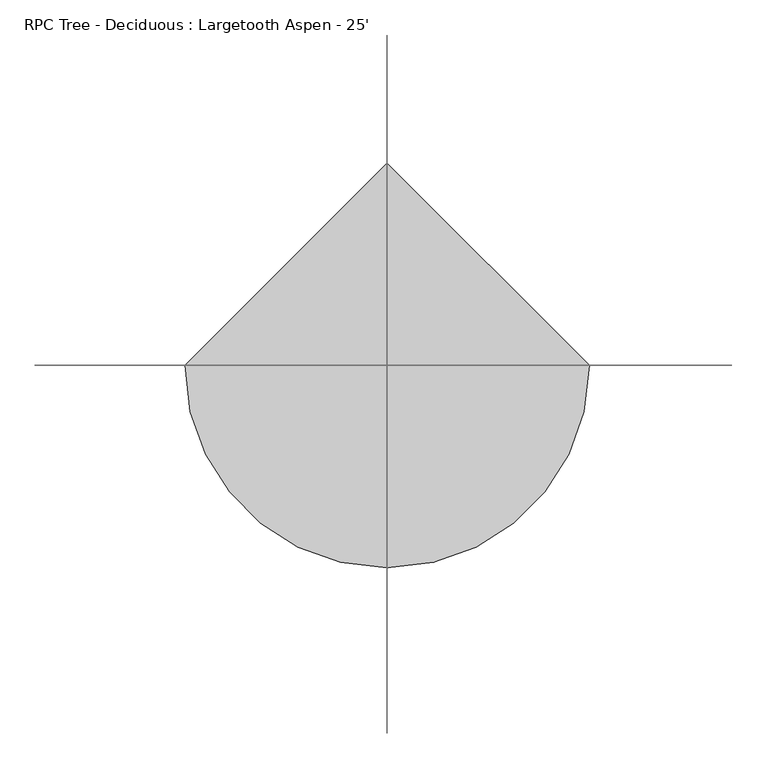
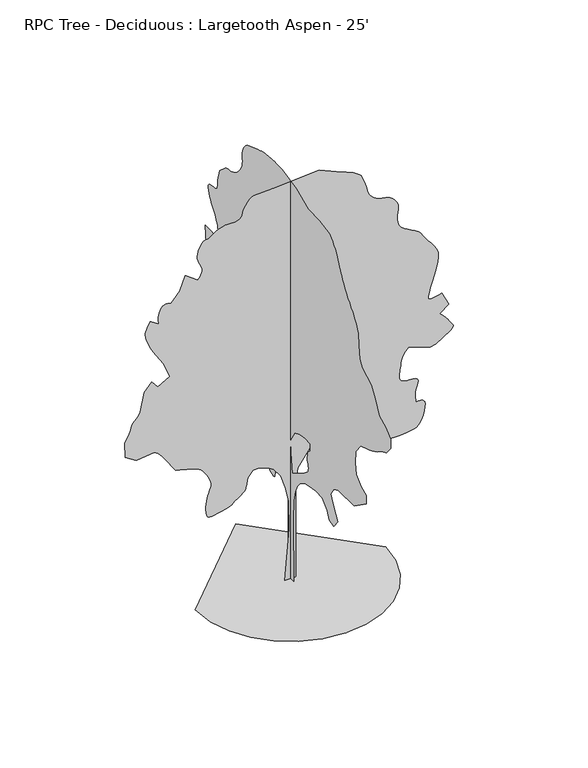
"""IFC4 building model written with IfcOpenShell, lengths in millimetres: geographic element geometry, RPC Tree - Deciduous : Largetooth Aspen - 25'."""

from ifc_helpers import new_model, si_unit, origin, place, context, project, spatial, triangles, source, transform, mapped, element, save


def rpc_tree_deciduous_largetooth_aspen_25_f6cd7aa4(model_context):
    return source(origin(), model_context, "Body", "Tessellation", [
        triangles([(93.1061447, 0.000407, 0.0055275), (-104.1894253, 0.000407, 0.0055275), (-22.9504001, 0.0003503, 951.6658939), (-34.5559031, 0.0003185, 1485.5251682), (-92.5836657, 0.0003019, 1764.061219), (-173.8237105, 0.0002874, 2007.7790462), (-301.4849952, 0.000277, 2181.8628971), (-405.9347789, 0.0002735, 2239.8916225), (-568.4133425, 0.0002701, 2297.9204933), (-684.470866, 0.0002701, 2297.9204933), (-765.710166, 0.000277, 2181.8628971), (-800.5284622, 0.000286, 2030.9895481), (-803.4037228, 0.000287, 2013.4305908), (-808.6158319, 0.0002881, 1994.9546837), (-818.4938627, 0.0002893, 1974.6550507), (-835.3797506, 0.0002907, 1951.6121258), (-861.6001705, 0.0002923, 1924.9168076), (-899.4969126, 0.0002942, 1893.6518555), (-951.4017385, 0.0002963, 1856.9058426), (-1000.9367964, 0.0002984, 1821.7851665), (-1035.041328, 0.0003, 1794.7824543), (-1061.0280413, 0.0003013, 1774.0764507), (-1086.2019407, 0.0003023, 1757.8357269), (-1117.8706472, 0.0003031, 1744.2340862), (-1163.3467958, 0.0003038, 1731.4425705), (-1229.9353912, 0.0003046, 1717.6377445), (-1303.2575146, 0.0003056, 1701.9735844), (-1364.6008633, 0.0003064, 1687.5234489), (-1414.7786144, 0.000307, 1678.356712), (-1454.6032185, 0.000307, 1678.5242889), (-1484.8875618, 0.0003062, 1692.0929375), (-1506.439444, 0.0003043, 1723.119096), (-1520.076693, 0.0003012, 1775.66647), (-1526.0305447, 0.0002975, 1838.229221), (-1525.0830734, 0.000294, 1896.7304466), (-1518.8575813, 0.0002907, 1951.3759483), (-1508.9769344, 0.0002877, 2002.3662952), (-1497.0669056, 0.0002848, 2049.9049633), (-1484.7505062, 0.0002822, 2094.1948471), (-1473.6532185, 0.0002797, 2135.4418934), (-1462.0149754, 0.0002776, 2171.5098953), (-1448.7511047, 0.0002758, 2202.2997311), (-1436.5031605, 0.000274, 2231.0600395), (-1427.9079002, 0.0002723, 2261.0397503), (-1425.6065872, 0.0002702, 2295.4845955), (-1432.2385952, 0.0002677, 2337.6435047), (-1450.4427166, 0.0002645, 2390.7649715), (-1477.2752357, 0.0002611, 2448.2171333), (-1507.353923, 0.000258, 2500.7976448), (-1539.6676483, 0.0002552, 2547.8968048), (-1573.1981598, 0.0002527, 2588.9178474), (-1606.9320019, 0.0002507, 2623.2079056), (-1639.8528122, 0.0002491, 2650.2080017), (-1670.950042, 0.0002479, 2669.3088707), (-1706.2051575, 0.000247, 2684.2184258), (-1751.2088058, 0.0002461, 2699.1535606), (-1804.330418, 0.0002453, 2714.0634064), (-1863.9491627, 0.0002444, 2728.9985413), (-1928.439703, 0.0002435, 2743.908387), (-1996.1788822, 0.0002426, 2758.8182327), (-2065.5412182, 0.0002417, 2773.7533676), (-2262.8354256, 0.0002244, 3063.8972855), (-2307.8392193, 0.0002208, 3124.7302002), (-2344.3134464, 0.0002181, 3169.7390808), (-2373.6809853, 0.0002162, 3201.539756), (-2397.3664581, 0.0002149, 3222.7742157), (-2416.7872204, 0.0002141, 3236.1091576), (-2433.3683304, 0.0002137, 3244.1609917), (-2448.5269981, 0.0002133, 3249.5711266), (-2773.4740242, 0.0002154, 3214.7732506), (-2970.7811668, 0.0002078, 3342.4334816), (-2982.3888885, 0.0001919, 3609.3616653), (-2960.1129227, 0.0001895, 3649.1127274), (-2938.5738304, 0.0001872, 3688.6606041), (-2918.4317459, 0.0001848, 3727.8273994), (-2900.4229614, 0.0001825, 3766.3590591), (-2885.2846413, 0.0001803, 3804.0779778), (-2873.6769196, 0.0001781, 3840.78097), (-2866.3363792, 0.000176, 3876.2901398), (-2854.8809738, 0.000174, 3909.843615), (-2833.1131165, 0.0001721, 3941.5934212), (-2804.8174599, 0.0001702, 3972.5051971), (-2773.8803947, 0.0001684, 4003.6457382), (-2744.1877304, 0.0001665, 4035.9798111), (-2719.5499901, 0.0001644, 4070.5745018), (-2703.8526924, 0.0001621, 4108.3951584), (-2634.2060715, 0.0001414, 4456.5779755), (-2494.950618, 0.0001324, 4607.4283607), (-2390.4982727, 0.00014, 4479.7681297), (-2169.9909473, 0.0001331, 4595.8459282), (-2286.0485435, 0.0001158, 4885.9645569), (-2471.7375, 9.85e-05, 5176.1084747), (-2494.0692764, 9.6e-05, 5217.3577011), (-2519.6494011, 9.3e-05, 5268.7673538), (-2546.0425575, 8.96e-05, 5326.2475662), (-2570.8076157, 8.6e-05, 5385.7596313), (-2591.5086777, 8.26e-05, 5443.2398438), (-2605.7325188, 7.95e-05, 5494.6494965), (-2611.0159172, 7.71e-05, 5535.8993042), (-2608.2980598, 7.5e-05, 5570.3669678), (-2600.7287544, 7.3e-05, 5604.2503647), (-2589.0701637, 7.1e-05, 5637.6006546), (-2574.1858978, 6.9e-05, 5670.544574), (-2556.863118, 6.71e-05, 5703.2088593), (-2537.9197975, 6.52e-05, 5735.6446701), (-2518.1611198, 6.32e-05, 5768.0037415), (-2367.2877708, 6.95e-05, 5663.5595352), (-2372.0934368, 6.75e-05, 5695.9697662), (-2375.8831764, 6.56e-05, 5728.8881058), (-2377.6407726, 6.35e-05, 5762.8226624), (-2376.3555313, 6.14e-05, 5798.2809631), (-2371.00891, 5.92e-05, 5835.7711166), (-2360.5873077, 5.68e-05, 5875.8018127), (-2344.077269, 5.42e-05, 5918.8799973), (-2322.4899239, 5.2e-05, 5956.5480469), (-2297.8569798, 5.05e-05, 5981.4145523), (-2270.6865452, 4.97e-05, 5995.6131042), (-2241.4867287, 4.93e-05, 6001.3028732), (-2210.7630226, 4.94e-05, 6000.5918701), (-2179.0257156, 4.97e-05, 5995.6131042), (-2146.7804455, 5.01e-05, 5988.501329), (-1995.9070965, 3.97e-05, 6162.5924469), (-1891.4573673, 2.45e-05, 6417.9129089), (-1670.950042, 3.42e-05, 6255.4298035), (-1648.8215961, 3.24e-05, 6285.3250717), (-1628.2145691, 3.06e-05, 6315.3988174), (-1610.6529957, 2.88e-05, 6345.8789337), (-1597.6609108, 2.69e-05, 6376.9683151), (-1590.7597332, 2.5e-05, 6408.8960175), (-1591.4684109, 2.31e-05, 6441.814357), (-1601.3160656, 2.1e-05, 6475.9523895), (-1617.3536041, 1.89e-05, 6510.877002), (-1634.407069, 1.68e-05, 6546.3864624), (-1650.6477928, 1.46e-05, 6583.140033), (-1664.2495789, 1.23e-05, 6621.7225616), (-1673.3859398, 9.9e-06, 6662.7183151), (-1676.2282082, 7.3e-06, 6706.761557), (-1670.950042, 4.4e-06, 6754.488295), (-1658.2957272, 1.5e-06, 6803.2306686), (-1640.7672913, -1.2e-06, 6848.9505524), (-1619.1798008, -3.6e-06, 6889.9968842), (-1594.3462875, -5.7e-06, 6924.7441818), (-1567.0742603, -7.3e-06, 6951.5663818), (-1538.1767509, -8.4e-06, 6968.8641632), (-1508.471442, -8.7e-06, 6974.9853012), (-1475.2102455, -9.2e-06, 6983.3417679), (-1435.6574272, -1.05e-05, 7004.9067307), (-1390.6206413, -1.23e-05, 7034.3706299), (-1340.9153904, -1.42e-05, 7066.4762283), (-1287.3545609, -1.59e-05, 7095.9401276), (-1230.7481323, -1.72e-05, 7117.504509), (-1171.9065931, -1.77e-05, 7125.861557), (-1111.9499331, -1.77e-05, 7125.5313446), (-1053.2124573, -1.77e-05, 7125.9882935), (-998.3307781, -1.79e-05, 7129.5188919), (-949.9463768, -1.85e-05, 7138.307309), (-910.695793, -1.94e-05, 7154.6138718), (-883.2205805, -2.1e-05, 7180.6744904), (-870.1599678, -2.32e-05, 7218.6983322), (-859.1973375, -2.62e-05, 7267.6691803), (-837.8816328, -2.94e-05, 7321.8984283), (-808.6488241, -3.27e-05, 7376.76194), (-773.9321205, -3.57e-05, 7427.5367477), (-736.1725794, -3.82e-05, 7469.5992966), (-697.8033371, -3.99e-05, 7498.2504547), (-661.2603642, -4.05e-05, 7508.8422501), (-324.6980224, -4.19e-05, 7532.0576935), (510.9103117, -4.54e-05, 7590.0965927), (928.7119898, -3.43e-05, 7404.3974625), (997.9725878, -3.27e-05, 7376.9148376), (1065.003162, -3.1e-05, 7348.7462082), (1127.5632969, -2.92e-05, 7319.1294113), (1183.4279829, -2.73e-05, 7287.4051849), (1230.3570225, -2.53e-05, 7252.8102036), (1266.1201012, -2.3e-05, 7214.6852051), (1288.4873405, -2.05e-05, 7172.2924438), (1303.3743679, -1.8e-05, 7130.6618454), (1318.0580647, -1.58e-05, 7093.7303787), (1332.3378616, -1.37e-05, 7059.0086609), (1346.0081028, -1.16e-05, 7024.0834671), (1358.8656029, -9.4e-06, 6986.5171555), (1370.7070312, -6.9e-06, 6943.8959198), (1381.3319641, -3.9e-06, 6893.7565384), (1397.2017803, -8e-07, 6841.9149353), (1423.0183731, 2e-06, 6795.9665771), (1455.9391834, 4.3e-06, 6756.1137772), (1493.1248497, 6.3e-06, 6722.5350128), (1531.7301968, 7.9e-06, 6695.4843384), (1568.915863, 9.2e-06, 6675.1134888), (1601.8392895, 1e-05, 6661.6259399), (1632.2912098, 1.04e-05, 6653.548526), (1663.5535458, 1.08e-05, 6648.1133926), (1695.0215378, 1.1e-05, 6643.6683151), (1726.0831593, 1.13e-05, 6638.6389709), (1756.1288544, 1.18e-05, 6631.3492996), (1784.5513927, 1.24e-05, 6620.2238159), (1810.7387478, 1.34e-05, 6603.6126205), (1836.0828403, 1.48e-05, 6581.0320221), (1861.4244621, 1.64e-05, 6553.8028702), (1885.3461124, 1.82e-05, 6522.9169647), (1906.4256397, 2.02e-05, 6489.3887787), (1923.2429272, 2.23e-05, 6454.2351105), (1934.3756779, 2.45e-05, 6418.4721771), (1938.4015949, 2.66e-05, 6383.0900345), (1934.8836411, 2.9e-05, 6341.7640686), (1927.3043072, 3.21e-05, 6289.6434128), (1920.1313438, 3.57e-05, 6230.2325043), (1917.8301762, 3.94e-05, 6166.9613663), (1924.8685547, 4.32e-05, 6103.2838577), (1945.7117592, 4.69e-05, 6042.6538376), (1984.8250694, 5.01e-05, 5988.501329), (2039.569693, 5.28e-05, 5943.162236), (2101.6243355, 5.51e-05, 5904.3256531), (2166.9277622, 5.72e-05, 5868.5371399), (2231.4183025, 5.94e-05, 5832.3166763), (2291.0370472, 6.18e-05, 5792.2609818), (2341.7227615, 6.46e-05, 5744.890036), (2379.4162457, 6.81e-05, 5686.7749786), (2417.9887459, 7.19e-05, 5621.9795151), (2469.1466698, 7.58e-05, 5556.3713104), (2525.585376, 7.98e-05, 5489.1376236), (2580.0024033, 8.4e-05, 5419.4657135), (2625.0618622, 8.83e-05, 5346.5422577), (2653.4845459, 9.29e-05, 5269.5800949), (2657.9549126, 9.78e-05, 5187.7164871), (2641.5719009, 0.0001035, 5093.1519104), (2615.0543335, 0.00011, 4983.9574127), (2582.4409172, 0.0001169, 4868.2862755), (2547.7697777, 0.0001237, 4754.2147499), (2515.1639191, 0.0001299, 4649.8972801), (2488.6361778, 0.000135, 4563.4609863), (2472.2607239, 0.0001386, 4502.9835732), (2471.4479828, 0.0001408, 4466.6872421), (2487.0816216, 0.000142, 4445.6050987), (2516.4161682, 0.0001425, 4437.2230522), (2556.710511, 0.0001424, 4438.9758522), (2605.2247009, 0.0001419, 4448.3482452), (2659.2248932, 0.000141, 4462.8008514), (2715.9685226, 0.00014, 4479.7681297), (2843.6287537, 0.0001552, 4224.4476677), (2681.1706467, 0.0001628, 4096.7874367), (2705.9862831, 0.0001642, 4074.3338654), (2730.6243141, 0.0001655, 4051.3466057), (2754.8559746, 0.000167, 4027.3692902), (2778.4777885, 0.0001685, 4001.8420692), (2801.2868614, 0.0001701, 3974.3085754), (2823.0802986, 0.0001719, 3944.2351204), (2843.6287537, 0.0001739, 3911.1135956), (2865.6250854, 0.0001758, 3878.8553902), (2888.8408195, 0.0001775, 3850.6614716), (2908.8050079, 0.000179, 3824.931356), (2921.0478653, 0.0001805, 3799.9886925), (2921.1240234, 0.0001821, 3774.2329971), (2904.5378265, 0.0001837, 3746.0643677), (2866.8441971, 0.0001857, 3713.8064529), (2611.523735, 0.000196, 3539.7150444), (2507.076622, 0.0001967, 3528.1073227), (2124.0931675, 0.0001891, 3655.7675537), (2096.88727, 0.0001908, 3628.2340599), (2070.5983223, 0.0001925, 3599.5829018), (2046.1355713, 0.0001943, 3568.6964149), (2024.4110252, 0.0001964, 3534.4319366), (2006.3439594, 0.0001987, 3495.74767), (1992.8439114, 0.0002013, 3451.4500832), (1984.8250694, 0.0002043, 3400.4470917), (1979.2422707, 0.0002073, 3350.9425552), (1972.8464401, 0.0002097, 3309.9723816), (1966.2475697, 0.0002118, 3274.6916862), (1960.0550697, 0.0002138, 3242.2305862), (1954.8784962, 0.0002157, 3209.7947754), (1951.3250793, 0.0002178, 3174.4887909), (1950.0068459, 0.0002203, 3133.5186172), (1959.0060059, 0.0002226, 3094.8599304), (1982.2191238, 0.0002242, 3067.1485405), (2013.9564308, 0.0002253, 3048.55578), (2048.5358608, 0.000226, 3037.3035599), (2080.2731678, 0.0002263, 3031.5123436), (2103.4861404, 0.0002265, 3029.3787529), (2112.4854458, 0.0002265, 3029.0738297), (2125.1752235, 0.0002264, 3029.9630196), (2157.148708, 0.0002264, 3030.4202591), (2199.274625, 0.0002266, 3027.2451622), (2242.4164684, 0.0002272, 3017.1614754), (2277.4354065, 0.0002284, 2996.942942), (2295.2001652, 0.0002304, 2963.2880196), (2286.5717674, 0.0002334, 2913.021611), (2265.7615551, 0.0002368, 2855.3635025), (2252.261507, 0.0002401, 2801.3633102), (2244.8497501, 0.0002431, 2750.4108971), (2242.3122597, 0.000246, 2701.871418), (2243.429924, 0.0002488, 2655.1864769), (2246.9833408, 0.0002515, 2609.7203568), (2251.7533985, 0.0002541, 2564.8385033), (2291.2047695, 0.0002539, 2569.2835808), (2328.629084, 0.0002538, 2570.4774033), (2361.9894024, 0.0002541, 2565.1434265), (2389.2612843, 0.000255, 2550.1065536), (2408.4128769, 0.0002567, 2522.0472198), (2417.4120369, 0.0002593, 2477.7574814), (2414.2319984, 0.0002631, 2413.9754734), (2401.476091, 0.0002675, 2341.0953289), (2383.2389774, 0.0002716, 2272.8811787), (2359.7236977, 0.0002752, 2211.166777), (2331.1309662, 0.0002784, 2157.7735245), (2297.6690552, 0.000281, 2114.5300884), (2259.536063, 0.0002829, 2083.2677525), (2216.9377911, 0.0002839, 2065.807917), (2176.9759861, 0.0002844, 2057.1795193), (2143.1075592, 0.0002848, 2050.7838341), (2110.049548, 0.0002851, 2046.0136311), (2072.5261116, 0.0002853, 2042.257029), (2025.2567585, 0.0002855, 2038.9092682), (1962.9659386, 0.0002857, 2035.3558514), (1880.3728695, 0.000286, 2030.9895481), (1790.6068371, 0.0002859, 2032.4449825), (1709.3674644, 0.0002851, 2045.4726757), (1635.2326, 0.0002838, 2068.1420769), (1566.7847431, 0.0002819, 2098.5255421), (1502.5989807, 0.0002798, 2134.6977528), (1441.2554867, 0.0002774, 2174.7255421), (1381.3319641, 0.0002749, 2216.6811207), (1126.0062698, 0.0002604, 2460.3989479), (859.0779408, 0.0002535, 2576.4465157), (545.7260645, 0.0002548, 2553.2563614), (394.8527518, 0.0002618, 2437.1885914), (290.4029863, 0.0002708, 2286.3152424), (127.9229058, 0.0002846, 2054.2026661), (93.1061447, 0.0003019, 1764.061219), (93.1061447, 0.0003392, 1137.3575392), (-0.0023708, 90.8437737, 1.11e-05), (-0.0023708, -94.8460457, 0.0), (-0.0023708, -83.2405405, 1160.5629541), (-0.0023708, -94.8460457, 1531.9435558), (-0.0023708, -141.2688208, 1729.2379086), (-0.0023708, -210.9025882, 1880.1112576), (-0.0023708, -303.7481383, 1996.1687084), (-0.0023708, -443.0162001, 2077.4080811), (-0.0023708, -559.0712165, 2100.6185829), (-0.0023708, -791.1838291, 2147.0420574), (-0.0023708, -988.4806526, 2135.4368065), (-0.0023708, -1139.3539289, 1984.5634575), (-0.0023708, -1208.987978, 1845.2955048), (-0.0023708, -1336.648209, 1798.8718849), (-0.0023708, -1475.9163071, 1972.9557358), (-0.0023708, -1325.0429581, 2205.0707829), (-0.0023708, -1255.4089817, 2367.5493828), (-0.0023708, -1336.648209, 2506.8150101), (-0.0023708, -1487.521558, 2576.4465157), (-0.0023708, -1974.9572124, 2576.4465157), (-0.0023708, -2357.9431377, 2843.3746994), (-0.0023708, -2357.9431377, 3005.8583862), (-0.0023708, -2195.4645378, 3075.479718), (-0.0023708, -2044.5913342, 3214.7476707), (-0.0023708, -2009.7755814, 3412.0548134), (-0.0023708, -2032.9860832, 3644.159832), (-0.0023708, -2183.8592869, 3841.466684), (-0.0023708, -2450.787616, 3934.3037498), (-0.0023708, -2495.4866318, 3951.778846), (-0.0023708, -2539.7763702, 3969.5332855), (-0.0023708, -2583.2536583, 3987.8975716), (-0.0023708, -2625.5191017, 4007.2016258), (-0.0023708, -2666.159063, 4027.6995026), (-0.0023708, -2704.7671715, 4049.7211235), (-0.0023708, -2740.9367661, 4073.5717026), (-0.0023708, -2775.734642, 4097.0920692), (-0.0023708, -2810.5580978, 4118.1742126), (-0.0023708, -2845.381263, 4137.223922), (-0.0023708, -2880.2047188, 4154.6484398), (-0.0023708, -2915.0025948, 4170.8535553), (-0.0023708, -2949.8260506, 4186.2459297), (-0.0023708, -2984.6495064, 4201.2319336), (-0.0023708, -3112.3097374, 4363.7156204), (-0.0023708, -3112.3097374, 4526.1993073), (-0.0023708, -2961.4337723, 4665.46726), (-0.0023708, -2764.1522095, 4769.9120476), (-0.0023708, -2636.4666893, 5013.6247879), (-0.0023708, -2508.8189575, 5199.3239182), (-0.0023708, -2230.2829067, 5350.1995926), (-0.0023708, -2149.0435341, 5477.860405), (-0.0023708, -2125.8305614, 5733.180867), (-0.0023708, -2102.6200596, 5942.0698608), (-0.0023708, -2077.7179459, 5994.1655182), (-0.0023708, -2052.6126469, 6045.3211166), (-0.0023708, -2027.0983612, 6094.647757), (-0.0023708, -2000.9769905, 6141.2315414), (-0.0023708, -1974.0453495, 6184.1824081), (-0.0023708, -1946.0953114, 6222.5364624), (-0.0023708, -1916.9309578, 6255.4298035), (-0.0023708, -1880.7588924, 6294.3169647), (-0.0023708, -1835.0490372, 6347.6061539), (-0.0023708, -1784.4624447, 6409.8360764), (-0.0023708, -1733.6777538, 6475.4948593), (-0.0023708, -1687.355872, 6539.1473694), (-0.0023708, -1650.170351, 6595.2811523), (-0.0023708, -1626.7896561, 6638.4104965), (-0.0023708, -1609.9062389, 6674.6559586), (-0.0023708, -1589.7741829, 6713.7465958), (-0.0023708, -1567.4070889, 6755.6568283), (-0.0023708, -1543.8256794, 6800.4366531), (-0.0023708, -1520.0386139, 6848.0360733), (-0.0023708, -1497.0642895, 6898.4806686), (-0.0023708, -1475.9163071, 6951.7698578), (-0.0023708, -1452.6372047, 7005.1352051), (-0.0023708, -1423.2671951, 7056.0623291), (-0.0023708, -1388.8223499, 7104.957019), (-0.0023708, -1350.3185955, 7152.2262268), (-0.0023708, -1308.7667713, 7198.2763229), (-0.0023708, -1265.188036, 7243.513678), (-0.0023708, -1220.5932289, 7288.3446625), (-0.0023708, -895.6335583, 7346.3585632), (-0.0023708, -547.4659656, 7357.9659943), (-0.0023708, -176.0855819, 7520.4496811), (-0.0023708, 264.9268161, 7613.2870377), (-0.0023708, 324.5456334, 7615.7252609), (-0.0023708, 383.7580439, 7617.8588516), (-0.0023708, 442.1602203, 7619.3825958), (-0.0023708, 499.3406327, 7619.9924423), (-0.0023708, 554.9005408, 7619.3825958), (-0.0023708, 608.4284509, 7617.2490051), (-0.0023708, 659.5204994, 7613.2870377), (-0.0023708, 708.649114, 7608.2065338), (-0.0023708, 756.9649876, 7602.5423447), (-0.0023708, 805.0801466, 7595.6340454), (-0.0023708, 853.6016762, 7586.8962067), (-0.0023708, 903.136734, 7575.7457245), (-0.0023708, 954.2948032, 7561.5215927), (-0.0023708, 1007.6881285, 7543.6657059), (-0.0023708, 1344.2529774, 7427.6129059), (-0.0023708, 1373.9607571, 7402.5429245), (-0.0023708, 1402.8557957, 7376.228833), (-0.0023708, 1430.1278229, 7347.5015167), (-0.0023708, 1454.9613361, 7315.141864), (-0.0023708, 1476.5488266, 7277.8801849), (-0.0023708, 1494.0772625, 7234.5479462), (-0.0023708, 1506.7315773, 7183.8748764), (-0.0023708, 1511.0952644, 7135.4627151), (-0.0023708, 1507.5418476, 7096.3970764), (-0.0023708, 1500.9454479, 7061.7770966), (-0.0023708, 1496.1727741, 7026.7507462), (-0.0023708, 1498.1031796, 6986.4659958), (-0.0023708, 1511.6032276, 6935.996402), (-0.0023708, 1541.5473301, 6870.5405136), (-0.0023708, 1582.5555828, 6804.0434097), (-0.0023708, 1625.189463, 6752.1768082), (-0.0023708, 1668.2270977, 6712.4769058), (-0.0023708, 1710.4546074, 6682.5298965), (-0.0023708, 1750.6525898, 6659.8987198), (-0.0023708, 1787.5994625, 6642.1439896), (-0.0023708, 1820.0833809, 6626.8024841), (-0.0023708, 1849.9258907, 6615.6775818), (-0.0023708, 1879.7682552, 6610.2418671), (-0.0023708, 1909.6107651, 6607.6257477), (-0.0023708, 1939.4557457, 6605.0346268), (-0.0023708, 1969.2981102, 6599.5739136), (-0.0023708, 1999.14062, 6588.4484299), (-0.0023708, 2028.9829845, 6568.7891647), (-0.0023708, 2203.0693062, 6417.9129089), (-0.0023708, 2272.7008118, 6197.4159027), (-0.0023708, 2270.435107, 6162.7197647), (-0.0023708, 2269.4877811, 6128.8613663), (-0.0023708, 2271.179393, 6096.6034515), (-0.0023708, 2276.8307922, 6066.8093399), (-0.0023708, 2287.7578869, 6040.2411942), (-0.0023708, 2305.2864681, 6017.7367538), (-0.0023708, 2330.7295372, 6000.1087601), (-0.0023708, 2366.121999, 5990.0250732), (-0.0023708, 2409.2282341, 5986.2404205), (-0.0023708, 2454.9736977, 5983.6754608), (-0.0023708, 2498.2855888, 5977.2491089), (-0.0023708, 2534.0819504, 5961.8820236), (-0.0023708, 2557.2947777, 5932.4942825), (-0.0023708, 2562.8319397, 5884.0565414), (-0.0023708, 2554.1452606, 5827.7448624), (-0.0023708, 2538.7528862, 5777.5287415), (-0.0023708, 2517.7724808, 5732.3931244), (-0.0023708, 2492.3292664, 5691.3217941), (-0.0023708, 2463.5359657, 5653.2979523), (-0.0023708, 2432.5073364, 5617.3059631), (-0.0023708, 2400.3636589, 5582.3046112), (-0.0023708, 2375.59613, 5540.0391678), (-0.0023708, 2351.4381569, 5497.9004608), (-0.0023708, 2328.49697, 5455.9402313), (-0.0023708, 2307.3844505, 5414.284053), (-0.0023708, 2288.7053581, 5373.0342453), (-0.0023708, 2273.0741901, 5332.2931274), (-0.0023708, 2261.0955608, 5292.1606934), (-0.0023708, 2254.8700687, 5254.4164856), (-0.0023708, 2255.3450397, 5220.3046143), (-0.0023708, 2261.4003387, 5189.2402313), (-0.0023708, 2271.9235336, 5160.614653), (-0.0023708, 2285.7971054, 5133.8174515), (-0.0023708, 2301.9032444, 5108.2399429), (-0.0023708, 2319.1244316, 5083.2716995), (-0.0023708, 2469.9977806, 5106.4871429), (-0.0023708, 2655.6942947, 5106.4871429), (-0.0023708, 2632.4788513, 4769.9120476), (-0.0023708, 2423.5741608, 4410.1467979), (-0.0023708, 2416.0988903, 4367.9066437), (-0.0023708, 2408.5195564, 4325.9967018), (-0.0023708, 2400.7370373, 4284.6710266), (-0.0023708, 2392.6495949, 4244.2848289), (-0.0023708, 2384.1559273, 4205.0927444), (-0.0023708, 2375.1567673, 4167.4246948), (-0.0023708, 2365.5479061, 4131.6106018), (-0.0023708, 2351.1663712, 4092.901046), (-0.0023708, 2330.0869892, 4047.8924561), (-0.0023708, 2305.5556377, 3998.8448685), (-0.0023708, 2280.8237171, 3947.9433243), (-0.0023708, 2259.134634, 3897.4737305), (-0.0023708, 2243.7397888, 3849.620256), (-0.0023708, 2237.885059, 3806.6435188), (-0.0023708, 2242.6221245, 3768.5435188), (-0.0023708, 2255.8859951, 3733.4915886), (-0.0023708, 2276.2542286, 3700.9796196), (-0.0023708, 2302.3069988, 3670.4995033), (-0.0023708, 2332.6244797, 3641.5181328), (-0.0023708, 2365.7840836, 3613.5782684), (-0.0023708, 2400.3636589, 3586.1462219), (-0.0023708, 2713.7079048, 3655.7675537), (-0.0023708, 2731.0053955, 3606.110701), (-0.0023708, 2747.5915924, 3556.834639), (-0.0023708, 2762.7552017, 3508.3968979), (-0.0023708, 2775.7599312, 3461.1529793), (-0.0023708, 2785.945356, 3415.5345428), (-0.0023708, 2792.5748932, 3371.9482498), (-0.0023708, 2794.9625381, 3330.8257599), (-0.0023708, 2781.5002785, 3291.6333847), (-0.0023708, 2746.9055878, 3253.2540413), (-0.0023708, 2699.9410126, 3215.103463), (-0.0023708, 2649.3188118, 3176.5209343), (-0.0023708, 2603.7768242, 3136.9477684), (-0.0023708, 2572.0523071, 3095.7235405), (-0.0023708, 2562.8319397, 3052.2895638), (-0.0023708, 2571.1886971, 3010.557518), (-0.0023708, 2585.6413033, 2974.3117653), (-0.0023708, 2605.1738319, 2942.6631157), (-0.0023708, 2628.7450676, 2914.6470932), (-0.0023708, 2655.3896622, 2889.3742172), (-0.0023708, 2684.0408203, 2865.9044289), (-0.0023708, 2713.7079048, 2843.3746994), (-0.0023708, 2783.3545258, 2611.2696808), (-0.0023708, 2716.5272095, 2608.9584846), (-0.0023708, 2651.6302986, 2607.7899513), (-0.0023708, 2590.5941986, 2608.8314575), (-0.0023708, 2535.3339088, 2613.225666), (-0.0023708, 2487.7955315, 2622.0902412), (-0.0023708, 2449.8987167, 2636.5428474), (-0.0023708, 2423.5741608, 2657.7008583), (-0.0023708, 2398.2655312, 2683.9137932), (-0.0023708, 2363.2136009, 2712.5649513), (-0.0023708, 2320.0387653, 2743.2479622), (-0.0023708, 2270.3665066, 2775.5823257), (-0.0023708, 2215.8225975, 2809.1102211), (-0.0023708, 2158.0326656, 2843.4508575), (-0.0023708, 2098.6169609, 2878.1981552), (-0.0023708, 2096.1482162, 2840.8347382), (-0.0023708, 2093.7783028, 2803.1919777), (-0.0023708, 2091.6141907, 2764.9143723), (-0.0023708, 2089.7523857, 2725.7219971), (-0.0023708, 2088.2969513, 2685.3360901), (-0.0023708, 2087.3496254, 2643.4008591), (-0.0023708, 2087.01171, 2599.6619591), (-0.0023708, 2085.4216908, 2554.0943916), (-0.0023708, 2079.9734768, 2509.3195084), (-0.0023708, 2069.6534672, 2469.0222588), (-0.0023708, 2053.4457355, 2436.8431183), (-0.0023708, 2030.3368263, 2416.4418926), (-0.0023708, 1999.3108131, 2411.4660336), (-0.0023708, 1959.3490082, 2425.5756374), (-0.0023708, 1914.2462379, 2451.7986008), (-0.0023708, 1868.5363827, 2480.4573166), (-0.0023708, 1822.3160934, 2511.1455597), (-0.0023708, 1775.6894337, 2543.4517273), (-0.0023708, 1728.7603214, 2576.9799133), (-0.0023708, 1681.6281693, 2611.3461296), (-0.0023708, 1634.3918083, 2646.0931366), (-0.0023708, 1355.8582283, 2727.3221901), (-0.0023708, 1077.3221775, 2634.4854149), (-0.0023708, 903.2383266, 2425.5756374), (-0.0023708, 925.671623, 2395.8678577), (-0.0023708, 948.4096247, 2366.9728191), (-0.0023708, 971.754784, 2339.7009373), (-0.0023708, 996.0142771, 2314.8672787), (-0.0023708, 1021.4930271, 2293.2799335), (-0.0023708, 1048.4931959, 2275.7513523), (-0.0023708, 1077.3221775, 2263.0970375), (-0.0023708, 1104.7973173, 2250.7806381), (-0.0023708, 1128.0078192, 2234.2021442), (-0.0023708, 1147.667375, 2214.0700882), (-0.0023708, 1164.4821917, 2191.0957638), (-0.0023708, 1179.1684319, 2165.9904648), (-0.0023708, 1192.4323025, 2139.4627235), (-0.0023708, 1204.984952, 2112.2238338), (-0.0023708, 1172.5694887, 2104.7129551), (-0.0023708, 1139.6486057, 2096.8974438), (-0.0023708, 1105.7091803, 2088.4722313), (-0.0023708, 1070.2508068, 2079.1326851), (-0.0023708, 1032.7604353, 2068.576498), (-0.0023708, 992.7325733, 2056.4962761), (-0.0023708, 949.6593304, 2042.5897121), (-0.0023708, 906.5885582, 2025.6403107), (-0.0023708, 866.5607689, 2005.0332836), (-0.0023708, 829.0703974, 1981.383419), (-0.0023708, 793.6094805, 1955.2951859), (-0.0023708, 759.6725985, 1927.3806107), (-0.0023708, 726.7517155, 1898.2467785), (-0.0023708, 694.3362522, 1868.5060066), (-0.0023708, 694.3362522, 1706.0274067), (-0.0023708, 652.3120005, 1679.1287579), (-0.0023708, 611.8117109, 1654.968314), (-0.0023708, 574.3543679, 1636.2916924), (-0.0023708, 541.4665134, 1625.8370979), (-0.0023708, 514.6695299, 1626.3450611), (-0.0023708, 495.4849088, 1640.556403), (-0.0023708, 485.4341414, 1671.2116539), (-0.0023708, 480.5294263, 1705.9588062), (-0.0023708, 476.0285382, 1733.1976959), (-0.0023708, 472.3404639, 1756.7815762), (-0.0023708, 469.8715739, 1780.5661709), (-0.0023708, 469.025768, 1808.4147617), (-0.0023708, 470.2094167, 1844.1778404), (-0.0023708, 473.8288905, 1891.7165085), (-0.0023708, 476.7727515, 1943.7229271), (-0.0023708, 476.0615667, 1990.8550793), (-0.0023708, 472.3074354, 2033.9283222), (-0.0023708, 466.1149355, 2073.7529263), (-0.0023708, 458.0961662, 2111.1417778), (-0.0023708, 448.8581763, 2146.9074726), (-0.0023708, 439.0131741, 2181.8578102), (-0.0023708, 241.7168229, 2193.4630611), (-0.0023708, 137.2665396, 1996.1687084), (-0.0023708, 79.2382684, 1659.6039322), (-0.0023708, 79.2382684, 1230.1970032), (-0.0023708, 79.2382684, 591.8879997), (-0.0022508, -48.4240337, 2030.9844612), (-0.0022508, -2.0012081, 2402.3651356), (-0.0022508, 9.6043397, 2622.8776932), (-0.0022508, -129.6633155, 2843.3746994), (-0.0022508, -280.5376365, 2913.021611), (-0.0022508, -454.621451, 2936.2117653), (-0.0022508, -617.0999783, 2936.2117653), (-0.0022508, -617.0999783, 2796.9691017), (-0.0022508, -535.8607146, 2727.3221901), (-0.0022508, -512.6502128, 2564.8385033), (-0.0022508, -522.5282799, 2554.7295273), (-0.0022508, -532.0024836, 2543.6043343), (-0.0022508, -540.6638735, 2530.4344986), (-0.0022508, -548.1085862, 2514.226767), (-0.0022508, -553.9277441, 2493.9573647), (-0.0022508, -557.717411, 2468.6158882), (-0.0022508, -559.0712165, 2437.1808884), (-0.0022508, -555.6879564, 2404.7324329), (-0.0022508, -546.2137527, 2376.5486881), (-0.0022508, -531.6646408, 2351.915744), (-0.0022508, -513.0540762, 2330.1250683), (-0.0022508, -491.4006014, 2310.4679832), (-0.0022508, -467.7151285, 2292.2308697), (-0.0022508, -443.0162001, 2274.7022884), (-1711.8591728, 0.0, 0.0031267), (-1666.6040863, -392.2441901, 0.0031033), (-1537.7144245, -752.4590126, 0.0030819), (-1335.5154293, -1070.3218781, 0.0030629), (-1070.3218781, -1335.5154293, 0.0030471), (-752.4590126, -1537.7144245, 0.0030351), (-392.2441901, -1666.6040863, 0.0030274), (7.5e-05, -1711.8591728, 0.0030247), (392.2441901, -1666.6040863, 0.0030274), (752.4590126, -1537.7144245, 0.0030351), (1070.3218781, -1335.5154293, 0.0030471), (1335.5154293, -1070.3218781, 0.0030629), (1537.7144245, -752.4590126, 0.0030819), (1666.6040863, -392.2441901, 0.0031033), (1711.8591728, 0.0001497, 0.0031267), (-0.0002251, 1711.8591728, 0.0032287)], [[122, 123, 124], [87, 88, 89], [1, 2, 3], [329, 1, 3], [329, 3, 4], [328, 329, 4], [328, 4, 5], [105, 106, 107], [327, 328, 5], [327, 5, 6], [104, 105, 107], [238, 239, 240], [238, 240, 241], [237, 238, 241], [236, 237, 241], [103, 104, 107], [86, 87, 89], [235, 236, 241], [102, 103, 107], [101, 102, 107], [100, 101, 107], [99, 100, 107], [98, 99, 107], [97, 98, 107], [96, 97, 107], [327, 6, 7], [326, 327, 7], [95, 96, 107], [70, 71, 72], [69, 70, 72], [69, 72, 73], [69, 73, 74], [69, 74, 75], [69, 75, 76], [69, 76, 77], [69, 77, 78], [94, 95, 107], [234, 235, 241], [93, 94, 107], [69, 78, 79], [69, 79, 80], [69, 80, 81], [69, 81, 82], [69, 82, 83], [69, 83, 84], [69, 84, 85], [68, 69, 85], [325, 326, 7], [325, 7, 8], [67, 68, 85], [92, 93, 107], [91, 92, 107], [60, 61, 62], [67, 85, 86], [67, 86, 89], [67, 89, 90], [66, 67, 90], [65, 66, 90], [64, 65, 90], [63, 64, 90], [62, 63, 90], [60, 62, 90], [59, 60, 90], [58, 59, 90], [57, 58, 90], [56, 57, 90], [55, 56, 90], [54, 55, 90], [53, 54, 90], [284, 285, 286], [283, 284, 286], [282, 283, 286], [282, 286, 287], [281, 282, 287], [280, 281, 287], [279, 280, 287], [279, 287, 288], [278, 279, 288], [277, 278, 288], [277, 288, 289], [276, 277, 289], [275, 276, 289], [275, 289, 290], [52, 53, 90], [325, 8, 9], [121, 122, 124], [275, 290, 291], [30, 31, 32], [29, 30, 32], [29, 32, 33], [28, 29, 33], [28, 33, 34], [27, 28, 34], [27, 34, 35], [27, 35, 36], [26, 27, 36], [26, 36, 37], [26, 37, 38], [25, 26, 38], [25, 38, 39], [24, 25, 39], [23, 24, 39], [22, 23, 39], [21, 22, 39], [20, 21, 39], [20, 39, 40], [20, 40, 41], [20, 41, 42], [19, 20, 42], [19, 42, 43], [18, 19, 43], [18, 43, 44], [17, 18, 44], [16, 17, 44], [15, 16, 44], [14, 15, 44], [13, 14, 44], [12, 13, 44], [11, 12, 44], [11, 44, 45], [11, 45, 46], [10, 11, 46], [10, 46, 47], [10, 47, 48], [10, 48, 49], [10, 49, 50], [10, 50, 51], [252, 253, 254], [251, 252, 254], [251, 254, 255], [250, 251, 255], [249, 250, 255], [249, 255, 256], [248, 249, 256], [247, 248, 256], [246, 247, 256], [245, 246, 256], [245, 256, 257], [245, 257, 258], [244, 245, 258], [243, 244, 258], [242, 243, 258], [241, 242, 258], [234, 241, 258], [233, 234, 258], [274, 275, 291], [324, 325, 9], [51, 52, 90], [10, 51, 90], [9, 10, 90], [324, 9, 90], [323, 324, 90], [323, 90, 91], [323, 91, 107], [323, 107, 108], [323, 108, 109], [323, 109, 110], [323, 110, 111], [323, 111, 112], [323, 112, 113], [323, 113, 114], [323, 114, 115], [323, 115, 116], [323, 116, 117], [323, 117, 118], [323, 118, 119], [323, 119, 120], [323, 120, 121], [323, 121, 124], [323, 124, 125], [323, 125, 126], [323, 126, 127], [323, 127, 128], [323, 128, 129], [322, 323, 129], [322, 129, 130], [167, 168, 169], [274, 291, 292], [296, 297, 298], [296, 298, 299], [295, 296, 299], [294, 295, 299], [294, 299, 300], [293, 294, 300], [293, 300, 301], [293, 301, 302], [293, 302, 303], [293, 303, 304], [293, 304, 305], [293, 305, 306], [293, 306, 307], [293, 307, 308], [293, 308, 309], [293, 309, 310], [293, 310, 311], [293, 311, 312], [293, 312, 313], [293, 313, 314], [293, 314, 315], [293, 315, 316], [293, 316, 317], [293, 317, 318], [293, 318, 319], [292, 293, 319], [274, 292, 319], [274, 319, 320], [274, 320, 321], [274, 321, 322], [273, 274, 322], [273, 322, 130], [272, 273, 130], [271, 272, 130], [270, 271, 130], [269, 270, 130], [268, 269, 130], [267, 268, 130], [266, 267, 130], [265, 266, 130], [264, 265, 130], [263, 264, 130], [262, 263, 130], [261, 262, 130], [260, 261, 130], [259, 260, 130], [258, 259, 130], [233, 258, 130], [232, 233, 130], [231, 232, 130], [230, 231, 130], [229, 230, 130], [228, 229, 130], [227, 228, 130], [226, 227, 130], [225, 226, 130], [224, 225, 130], [223, 224, 130], [222, 223, 130], [221, 222, 130], [220, 221, 130], [219, 220, 130], [218, 219, 130], [217, 218, 130], [216, 217, 130], [215, 216, 130], [214, 215, 130], [213, 214, 130], [212, 213, 130], [211, 212, 130], [210, 211, 130], [209, 210, 130], [208, 209, 130], [207, 208, 130], [206, 207, 130], [205, 206, 130], [204, 205, 130], [203, 204, 130], [202, 203, 130], [201, 202, 130], [200, 201, 130], [199, 200, 130], [198, 199, 130], [197, 198, 130], [196, 197, 130], [195, 196, 130], [194, 195, 130], [193, 194, 130], [192, 193, 130], [191, 192, 130], [190, 191, 130], [189, 190, 130], [188, 189, 130], [187, 188, 130], [186, 187, 130], [185, 186, 130], [184, 185, 130], [183, 184, 130], [182, 183, 130], [181, 182, 130], [180, 181, 130], [179, 180, 130], [178, 179, 130], [177, 178, 130], [176, 177, 130], [175, 176, 130], [174, 175, 130], [173, 174, 130], [172, 173, 130], [171, 172, 130], [170, 171, 130], [169, 170, 130], [167, 169, 130], [167, 130, 131], [167, 131, 132], [167, 132, 133], [167, 133, 134], [167, 134, 135], [167, 135, 136], [164, 165, 166], [164, 166, 167], [163, 164, 167], [162, 163, 167], [161, 162, 167], [160, 161, 167], [159, 160, 167], [158, 159, 167], [143, 144, 145], [142, 143, 145], [141, 142, 145], [140, 141, 145], [140, 145, 146], [139, 140, 146], [138, 139, 146], [137, 138, 146], [136, 137, 146], [136, 146, 147], [136, 147, 148], [136, 148, 149], [136, 149, 150], [136, 150, 151], [136, 151, 152], [136, 152, 153], [136, 153, 154], [136, 154, 155], [136, 155, 156], [157, 158, 167], [157, 167, 136], [157, 136, 156], [634, 330, 635], [633, 634, 635], [632, 633, 635], [631, 632, 635], [540, 541, 542], [592, 593, 594], [494, 495, 496], [635, 330, 331], [635, 331, 332], [635, 332, 333], [635, 333, 334], [635, 334, 335], [658, 635, 335], [658, 335, 336], [658, 336, 337], [658, 337, 338], [540, 542, 543], [657, 658, 338], [631, 635, 636], [630, 631, 636], [518, 519, 520], [656, 657, 338], [656, 338, 339], [655, 656, 339], [654, 655, 339], [653, 654, 339], [540, 543, 544], [539, 540, 544], [518, 520, 521], [539, 544, 545], [538, 539, 545], [538, 545, 546], [538, 546, 547], [538, 547, 548], [537, 538, 548], [537, 548, 549], [536, 537, 549], [536, 549, 550], [536, 550, 551], [535, 536, 551], [535, 551, 552], [534, 535, 552], [493, 494, 496], [493, 496, 497], [343, 344, 345], [342, 343, 345], [341, 342, 345], [340, 341, 345], [340, 345, 346], [534, 552, 553], [533, 534, 553], [518, 521, 522], [350, 351, 352], [349, 350, 352], [349, 352, 353], [348, 349, 353], [533, 553, 554], [652, 653, 339], [518, 522, 523], [518, 523, 524], [533, 554, 555], [532, 533, 555], [518, 524, 525], [518, 525, 526], [518, 526, 527], [518, 527, 528], [518, 528, 529], [518, 529, 530], [518, 530, 531], [518, 531, 532], [518, 532, 555], [517, 518, 555], [516, 517, 555], [515, 516, 555], [607, 608, 609], [591, 592, 594], [591, 594, 595], [590, 591, 595], [590, 595, 596], [589, 590, 596], [588, 589, 596], [588, 596, 597], [587, 588, 597], [586, 587, 597], [586, 597, 598], [585, 586, 598], [585, 598, 599], [584, 585, 599], [584, 599, 600], [583, 584, 600], [583, 600, 601], [582, 583, 601], [514, 515, 555], [643, 644, 645], [630, 636, 637], [629, 630, 637], [581, 582, 601], [581, 601, 602], [348, 353, 354], [580, 581, 602], [580, 602, 603], [579, 580, 603], [651, 652, 339], [651, 339, 340], [651, 340, 346], [650, 651, 346], [649, 650, 346], [649, 346, 347], [648, 649, 347], [647, 648, 347], [646, 647, 347], [372, 373, 374], [371, 372, 374], [370, 371, 374], [369, 370, 374], [369, 374, 375], [368, 369, 375], [367, 368, 375], [366, 367, 375], [365, 366, 375], [364, 365, 375], [363, 364, 375], [362, 363, 375], [361, 362, 375], [360, 361, 375], [359, 360, 375], [358, 359, 375], [357, 358, 375], [356, 357, 375], [356, 375, 376], [356, 376, 377], [356, 377, 378], [645, 646, 347], [643, 645, 347], [642, 643, 347], [641, 642, 347], [641, 347, 348], [641, 348, 354], [641, 354, 355], [607, 609, 610], [513, 514, 555], [579, 603, 604], [607, 610, 611], [607, 611, 612], [607, 612, 613], [607, 613, 614], [607, 614, 615], [607, 615, 616], [607, 616, 617], [607, 617, 618], [607, 618, 619], [607, 619, 620], [607, 620, 621], [607, 621, 622], [607, 622, 623], [607, 623, 624], [606, 607, 624], [606, 624, 625], [605, 606, 625], [605, 625, 626], [604, 605, 626], [579, 604, 626], [579, 626, 627], [579, 627, 628], [579, 628, 629], [579, 629, 637], [578, 579, 637], [578, 637, 638], [355, 356, 378], [641, 355, 378], [641, 378, 379], [640, 641, 379], [639, 640, 379], [639, 379, 380], [639, 380, 381], [639, 381, 382], [639, 382, 383], [639, 383, 384], [639, 384, 385], [639, 385, 386], [639, 386, 387], [639, 387, 388], [639, 388, 389], [639, 389, 390], [639, 390, 391], [639, 391, 392], [639, 392, 393], [639, 393, 394], [639, 394, 395], [638, 639, 395], [578, 638, 395], [577, 578, 395], [577, 395, 396], [577, 396, 397], [577, 397, 398], [577, 398, 399], [577, 399, 400], [577, 400, 401], [577, 401, 402], [577, 402, 403], [577, 403, 404], [577, 404, 405], [577, 405, 406], [577, 406, 407], [577, 407, 408], [577, 408, 409], [577, 409, 410], [577, 410, 411], [577, 411, 412], [577, 412, 413], [577, 413, 414], [577, 414, 415], [577, 415, 416], [577, 416, 417], [577, 417, 418], [577, 418, 419], [577, 419, 420], [577, 420, 421], [577, 421, 422], [577, 422, 423], [577, 423, 424], [577, 424, 425], [577, 425, 426], [577, 426, 427], [577, 427, 428], [577, 428, 429], [577, 429, 430], [577, 430, 431], [577, 431, 432], [577, 432, 433], [577, 433, 434], [566, 567, 568], [566, 568, 569], [565, 566, 569], [564, 565, 569], [564, 569, 570], [563, 564, 570], [563, 570, 571], [562, 563, 571], [562, 571, 572], [561, 562, 572], [560, 561, 572], [560, 572, 573], [559, 560, 573], [559, 573, 574], [558, 559, 574], [558, 574, 575], [557, 558, 575], [556, 557, 575], [556, 575, 576], [555, 556, 576], [513, 555, 576], [513, 576, 577], [512, 513, 577], [511, 512, 577], [470, 471, 472], [469, 470, 472], [468, 469, 472], [468, 472, 473], [467, 468, 473], [467, 473, 474], [467, 474, 475], [466, 467, 475], [466, 475, 476], [466, 476, 477], [465, 466, 477], [465, 477, 478], [465, 478, 479], [464, 465, 479], [464, 479, 480], [464, 480, 481], [464, 481, 482], [463, 464, 482], [456, 457, 458], [456, 458, 459], [456, 459, 460], [510, 511, 577], [463, 482, 483], [455, 456, 460], [454, 455, 460], [453, 454, 460], [452, 453, 460], [451, 452, 460], [450, 451, 460], [450, 460, 461], [449, 450, 461], [449, 461, 462], [463, 483, 484], [492, 493, 497], [448, 449, 462], [447, 448, 462], [491, 492, 497], [462, 463, 484], [447, 462, 484], [447, 484, 485], [446, 447, 485], [446, 485, 486], [445, 446, 486], [445, 486, 487], [444, 445, 487], [444, 487, 488], [491, 497, 498], [509, 510, 577], [491, 498, 499], [491, 499, 500], [490, 491, 500], [490, 500, 501], [490, 501, 502], [490, 502, 503], [490, 503, 504], [490, 504, 505], [490, 505, 506], [490, 506, 507], [490, 507, 508], [490, 508, 509], [490, 509, 577], [489, 490, 577], [488, 489, 577], [444, 488, 577], [443, 444, 577], [442, 443, 577], [441, 442, 577], [440, 441, 577], [435, 436, 437], [434, 435, 437], [434, 437, 438], [434, 438, 439], [577, 434, 439], [440, 577, 439], [673, 674, 659], [672, 673, 659], [672, 659, 660], [671, 672, 660], [671, 660, 661], [671, 661, 662], [670, 671, 662], [669, 670, 662], [669, 662, 663], [669, 663, 664], [669, 664, 665], [669, 665, 666], [669, 666, 667], [669, 667, 668]], closed=False),
    ])


if __name__ == "__main__":
    model = new_model("IFC4")
    model_context = context("Model", 3, world=origin())
    ifc_project = project(units=[si_unit("LENGTHUNIT", "METRE", prefix="MILLI")], contexts=[model_context])
    site = spatial("IfcSite", under=ifc_project)
    building = spatial("IfcBuilding", under=site)
    placement = place(None, origin())
    rpc_tree_deciduous_largetooth_aspen_25_shape = rpc_tree_deciduous_largetooth_aspen_25_f6cd7aa4(model_context)
    element("IfcGeographicElement", 1, ObjectType="RPC Tree - Deciduous : Largetooth Aspen - 25'", at=placement, inside=building, context=model_context, shape_type="MappedRepresentation", body=[
        mapped(rpc_tree_deciduous_largetooth_aspen_25_shape, transform((0.0, 0.0, 0.0), x_axis=(1.0, 0.0, 0.0), y_axis=(0.0, 1.0, 0.0), z_axis=(0.0, 0.0, 1.0))),
    ])
    save(model, "model.ifc")

# Revit data of these elements
# Type "RPC Tree - Deciduous : Largetooth Aspen - 25'"
#   built-in parameter 1005198 = "{2, 15},{39, RPC-16-G0VG-J3PX-MQ0P-J000-ST1L-LVER-AU},{1, 0},{1, 0},{2, 35},{1, 8},{5, Color},{1, 0},{1, 0},{3, 0.8},{3, 0.8},{3, 0.8},{1, 8},{7, BBoxMin},{1, 0},{1, 0},{1, 0},{1, 0},{1, 0},{1, 8},{7, BBoxMax},{1, 0},{1, 0},{1, 0},{1, 0},{1, 0},{2, 11},{9, RPCTypeId},{1, 0},{1, 0},{39, RPC-16-G0VG-J3PX-MQ0P-J000-ST1L-LVER-AU},{1, 6},{14, RPCPlantHeight},{1, 0},{1, 0},{2, 25},{2, 11},{7, keyword},{1, 0},{1, 0},{178, :Geometry:RPC:Largetooth Aspen:Populus grandidentata:similar in form and aspect to trembling aspen; range does not extend as far west:east:or north; usually found on drier sites.},{2, 11},{8, category},{1, 0},{1, 0},{16, :Trees [General]},{2, 11},{12, LocalizedUID},{1, 0},{1, 0},{16, Largetooth Aspen},{2, 14},{6, Height},{1, 0},{1, 0},{2, 25},{1, 2},{16, Cast Reflections},{1, 0},{1, 0},{1, 0},{1, 2},{12, Cast Shadows},{1, 0},{1, 0},{1, 1},{1, 2},{9, Lock View},{1, 0},{1, 0},{1, 0},{1, 4},{5, ViewC},{1, 0},{1, 0},{1, 0},{2, 11},{20, AdvancedUIDefinition},{1, 0},{1, 0},{0, },{2, 11},{10, AssetLibID},{1, 0},{1, 0},{36, 4D3F6E72-3F99-4203-98E9-AF80B3C7A7A4},{2, 11},{10, BaseSchema},{1, 0},{1, 0},{9, RPCSchema},{2, 11},{12, ExchangeGUID},{1, 0},{1, 0},{0, },{1, 2},{6, Hidden},{1, 0},{1, 0},{1, 0},{1, 4},{11, RPCCategory},{1, 0},{1, 0},{1, 0},{2, 11},{8, RPCImage},{1, 0},{1, 0},{0, },{1, 4},{13, SchemaVersion},{1, 0},{1, 0},{1, 4},{2, 11},{12, UIDefinition},{1, 0},{1, 0},{0, },{2, 11},{6, UIName},{1, 0},{1, 0},{39, RPC-16-G0VG-J3PX-MQ0P-J000-ST1L-LVER-AU},{2, 11},{11, VersionGUID},{1, 0},{1, 0},{9, RPCSchema},{2, 11},{9, assettype},{1, 0},{1, 0},{11, RPCGeometry},{2, 11},{11, description},{1, 0},{1, 0},{0, },{2, 11},{9, localname},{1, 0},{1, 0},{3, RPC},{2, 11},{9, localtype},{1, 0},{1, 0},{3, RPC},{1, 4},{8, revision},{1, 0},{1, 0},{1, 1},{2, 11},{9, thumbnail},{1, 0},{1, 0},{0, },{1, 4},{7, version},{1, 0},{1, 0},{1, 1},{1, 2},{20, RPC_Cast Reflections},{1, 0},{1, 0},{1, 1},{1, 2},{16, RPC_Cast Shadows},{1, 0},{1, 0},{1, 1},{1, 2},{13, RPC_Lock View},{1, 0},{1, 0},{1, 0},{1, 4},{9, RPC_ViewC},{1, 0},{1, 0},{1, 0},{21, assetlibrary_base.fbx},{1, 5},"
#   built-in parameter 1005195 = "RPC-16-G0VG-J3PX-MQ0P-J000-ST1L-LVER-AU"
#   Type Comments = "Largetooth Aspen"
#   Assembly Code = "G2050500"
#   Height = 25' - 0"
#   Default Elevation = 0
